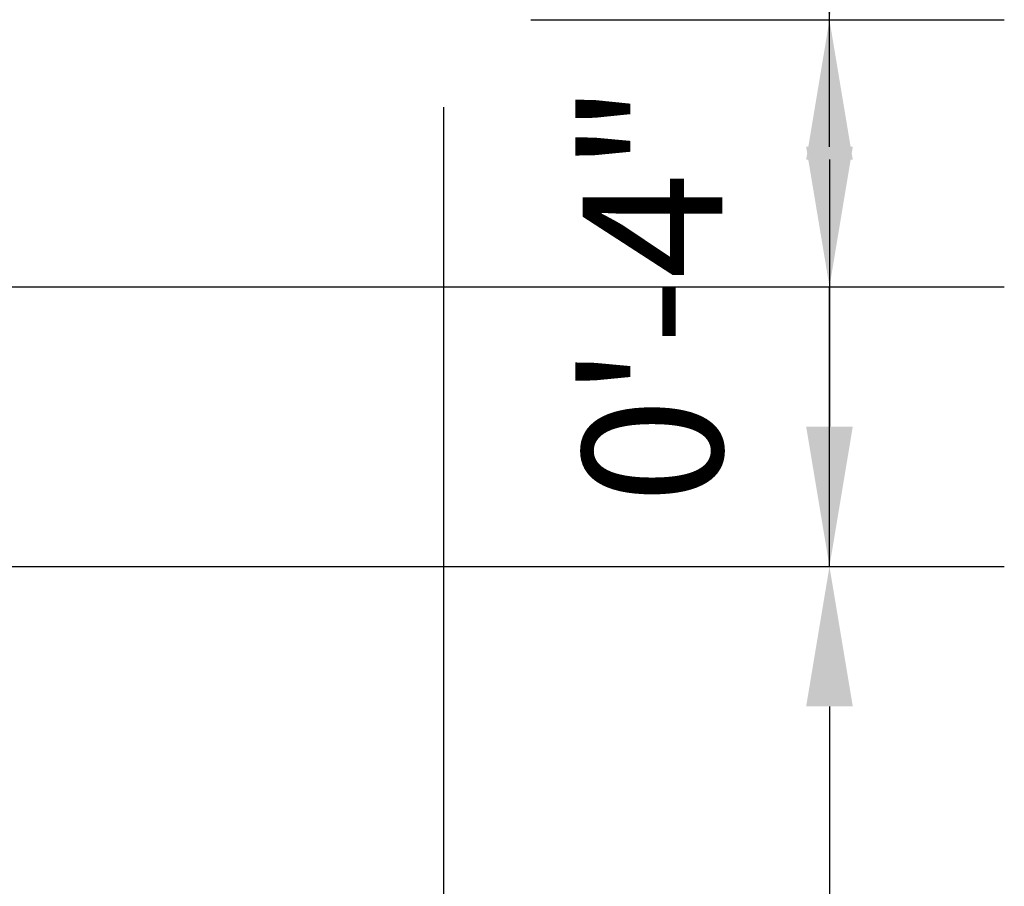
# Model space of a CAD drawing. Units: millimetres. Extents: x 7894 to 8038, y 6851 to 6951.
# Tile 36 of 49: x 7968.188 to 7975.227, y 6916.434 to 6922.628. Entities that reach past the tile are written whole.
import ezdxf

# ---------------------------------------------------------------- set-up
doc = ezdxf.new("R2010")
doc.units = ezdxf.units.MM
doc.layers.add('A-ANNO-DIMS', color=2, linetype='Continuous', lineweight=18)
doc.styles.get("Standard").update_dxf_attribs({"font": 'arial.ttf'})
doc.dimstyles.new('ISO-25', dxfattribs={"dimtxt": 1, "dimasz": 1, "dimexe": 1.25, "dimexo": 0.625, "dimtad": 1, "dimdec": 0, "dimlunit": 4, "dimtxsty": 'Standard', "dimcen": 2.5, "dimclrt": 1, "dimadec": 0, "dimazin": 0, "dimtfac": 1, "dimtdec": 0, "dimtmove": 0, "dimatfit": 3, "dimfxl": 1, "dimarcsym": 0})

# ---------------------------------------------------------------- blocks, each defined once
blk = doc.blocks.new('*D23')
at = {"layer": 'A-ANNO-DIMS', "color": 0, "lineweight": -2, "transparency": 16777216}
for p, q in [((7940.0888, 6907.098), (7940.0888, 6947.7928)), ((7971.9356, 6928.989), (7971.9356, 6947.7928)), ((7941.0888, 6946.5428), (7970.9356, 6946.5428))]:
    blk.add_line(p, q, dxfattribs=at)
at = {"layer": 'A-ANNO-DIMS', "color": 0, "transparency": 16777216}
for points in [[(7941.0888, 6946.7095), (7941.0888, 6946.3762), (7940.0888, 6946.5428)], [(7970.9356, 6946.7095), (7970.9356, 6946.3762), (7971.9356, 6946.5428)]]:
    blk.add_solid(points, dxfattribs=at)
at = {"layer": 'Defpoints', "color": 0, "transparency": 16777216}
for p in [(7971.9356, 6946.5428), (7971.9356, 6928.364), (7940.0888, 6906.473)]:
    blk.add_point(p, dxfattribs=at)
at = {"layer": 'A-ANNO-DIMS', "color": 1, "transparency": 16777216, "insert": (7956.0122, 6947.6784), "char_height": 1, "attachment_point": 5}
blk.add_mtext('2\'-8"', dxfattribs=at)
blk = doc.blocks.new('*D26')
at = {"layer": 'A-ANNO-DIMS', "color": 0, "lineweight": -2, "transparency": 16777216}
for p, q in [((7950.9654, 6918.7198), (7975.2272, 6918.7198)), ((7973.9772, 6917.7198), (7973.9772, 6907.4734)), ((7964.9658, 6906.4734), (7975.2272, 6906.4734))]:
    blk.add_line(p, q, dxfattribs=at)
at = {"layer": 'A-ANNO-DIMS', "color": 0, "transparency": 16777216}
for points in [[(7973.8105, 6917.7198), (7974.1439, 6917.7198), (7973.9772, 6918.7198)], [(7973.8105, 6907.4734), (7974.1439, 6907.4734), (7973.9772, 6906.4734)]]:
    blk.add_solid(points, dxfattribs=at)
at = {"layer": 'Defpoints', "color": 0, "transparency": 16777216}
for p in [(7950.3404, 6918.7198), (7964.3408, 6906.4734), (7973.9772, 6906.4734)]:
    blk.add_point(p, dxfattribs=at)
at = {"layer": 'A-ANNO-DIMS', "color": 1, "transparency": 16777216, "insert": (7972.8416, 6912.5966), "char_height": 1, "attachment_point": 5, "rotation": 90}
blk.add_mtext('1\'-0"', dxfattribs=at)
blk = doc.blocks.new('*D27')
at = {"layer": 'A-ANNO-DIMS', "color": 0, "lineweight": -2, "transparency": 16777216}
for p, q in [((7971.8421, 6922.6283), (7975.2272, 6922.6283)), ((7973.9772, 6921.6283), (7973.9772, 6919.7198)), ((7950.9654, 6918.7198), (7975.2272, 6918.7198))]:
    blk.add_line(p, q, dxfattribs=at)
at = {"layer": 'A-ANNO-DIMS', "color": 0, "transparency": 16777216}
for points in [[(7973.8105, 6921.6283), (7974.1439, 6921.6283), (7973.9772, 6922.6283)], [(7973.8105, 6919.7198), (7974.1439, 6919.7198), (7973.9772, 6918.7198)]]:
    blk.add_solid(points, dxfattribs=at)
at = {"layer": 'Defpoints', "color": 0, "transparency": 16777216}
for p in [(7971.2171, 6922.6283), (7950.3404, 6918.7198), (7973.9772, 6918.7198)]:
    blk.add_point(p, dxfattribs=at)
at = {"layer": 'A-ANNO-DIMS', "color": 1, "transparency": 16777216, "insert": (7972.8416, 6920.6741), "char_height": 1, "attachment_point": 5, "rotation": 90}
blk.add_mtext('0\'-4"', dxfattribs=at)
blk = doc.blocks.new('*D28')
at = {"layer": 'A-ANNO-DIMS', "color": 0, "lineweight": -2, "transparency": 16777216}
for p, q in [((7960.8854, 6936.8804), (7975.2272, 6936.8804)), ((7973.9772, 6935.8804), (7973.9772, 6923.6283)), ((7971.8421, 6922.6283), (7975.2272, 6922.6283))]:
    blk.add_line(p, q, dxfattribs=at)
at = {"layer": 'A-ANNO-DIMS', "color": 0, "transparency": 16777216}
for points in [[(7973.8105, 6935.8804), (7974.1439, 6935.8804), (7973.9772, 6936.8804)], [(7973.8105, 6923.6283), (7974.1439, 6923.6283), (7973.9772, 6922.6283)]]:
    blk.add_solid(points, dxfattribs=at)
at = {"layer": 'Defpoints', "color": 0, "transparency": 16777216}
for p in [(7960.2604, 6936.8804), (7971.2171, 6922.6283), (7973.9772, 6922.6283)]:
    blk.add_point(p, dxfattribs=at)
at = {"layer": 'A-ANNO-DIMS', "color": 1, "transparency": 16777216, "insert": (7972.8351, 6929.7543), "char_height": 1, "attachment_point": 5, "rotation": 90}
blk.add_mtext('1\'-2 1/2"', dxfattribs=at)
blk = doc.blocks.new('*D31')
at = {"layer": 'A-ANNO-DIMS', "color": 0, "lineweight": -2, "transparency": 16777216}
for p, q in [((7973.9772, 6921.7198), (7973.9772, 6926.628)), ((7949.8107, 6920.7198), (7975.2272, 6920.7198)), ((7973.9772, 6918.7198), (7973.9772, 6920.7198)), ((7950.9654, 6918.7198), (7975.2272, 6918.7198)), ((7973.9772, 6917.7198), (7973.9772, 6916.7198))]:
    blk.add_line(p, q, dxfattribs=at)
at = {"layer": 'A-ANNO-DIMS', "color": 0, "transparency": 16777216}
for points in [[(7973.8105, 6921.7198), (7974.1439, 6921.7198), (7973.9772, 6920.7198)], [(7973.8105, 6917.7198), (7974.1439, 6917.7198), (7973.9772, 6918.7198)]]:
    blk.add_solid(points, dxfattribs=at)
at = {"layer": 'Defpoints', "color": 0, "transparency": 16777216}
for p in [(7949.1857, 6920.7198), (7973.9772, 6920.7198), (7950.3404, 6918.7198)]:
    blk.add_point(p, dxfattribs=at)
at = {"layer": 'A-ANNO-DIMS', "color": 1, "transparency": 16777216, "insert": (7972.8416, 6924.6739), "char_height": 1, "attachment_point": 5, "rotation": 90}
blk.add_mtext('0\'-2"', dxfattribs=at)
blk = doc.blocks.new('*D34')
at = {"layer": 'A-ANNO-DIMS', "color": 0, "lineweight": -2, "transparency": 16777216}
for p, q in [((7971.2171, 6922.0033), (7971.2171, 6903.2865)), ((7964.3408, 6905.8484), (7964.3408, 6903.2865)), ((7965.3408, 6904.5365), (7970.2171, 6904.5365))]:
    blk.add_line(p, q, dxfattribs=at)
at = {"layer": 'A-ANNO-DIMS', "color": 0, "transparency": 16777216}
for points in [[(7965.3408, 6904.7032), (7965.3408, 6904.3699), (7964.3408, 6904.5365)], [(7970.2171, 6904.7032), (7970.2171, 6904.3699), (7971.2171, 6904.5365)]]:
    blk.add_solid(points, dxfattribs=at)
at = {"layer": 'Defpoints', "color": 0, "transparency": 16777216}
for p in [(7971.2171, 6922.6283), (7964.3408, 6906.4734), (7971.2171, 6904.5365)]:
    blk.add_point(p, dxfattribs=at)
at = {"layer": 'A-ANNO-DIMS', "color": 1, "transparency": 16777216, "insert": (7967.779, 6905.6721), "char_height": 1, "attachment_point": 5}
blk.add_mtext('0\'-7"', dxfattribs=at)

msp = doc.modelspace()

# ---------------------------------------------------------------- dimensions: what is measured, and where the dimension line sits
at = {"layer": 'A-ANNO-DIMS'}
for base, p1, p2, picture, middle in [((7971.9356, 6946.5428), (7940.0888, 6906.473), (7971.9356, 6928.364), '*D23', (7956.0122, 6947.6784)), ((7971.2171, 6904.5365), (7964.3408, 6906.4734), (7971.2171, 6922.6283), '*D34', (7967.779, 6905.6721))]:
    dim = msp.add_linear_dim(base=base, p1=p1, p2=p2, dimstyle='ISO-25', override={"dimdec": 1, "dimlfac": 1, "dimrnd": 0, "dimzin": 1, "dimdsep": 46, "dimlunit": 4, "dimfrac": 2}, dxfattribs=at)
    dim.commit()
    dim.dimension.update_dxf_attribs({"geometry": picture, "text_midpoint": middle})
for base, p1, p2, picture, middle in [((7973.9772, 6922.6283), (7960.2604, 6936.8804), (7971.2171, 6922.6283), '*D28', (7972.8351, 6929.7543)), ((7973.9772, 6920.7198), (7950.3404, 6918.7198), (7949.1857, 6920.7198), '*D31', (7972.8416, 6924.6739)), ((7973.9772, 6918.7198), (7971.2171, 6922.6283), (7950.3404, 6918.7198), '*D27', (7972.8416, 6920.6741)), ((7973.9772, 6906.4734), (7950.3404, 6918.7198), (7964.3408, 6906.4734), '*D26', (7972.8416, 6912.5966))]:
    dim = msp.add_linear_dim(base=base, p1=p1, p2=p2, angle=90, dimstyle='ISO-25', override={"dimdec": 1, "dimlfac": 1, "dimrnd": 0, "dimzin": 1, "dimdsep": 46, "dimlunit": 4, "dimfrac": 2}, dxfattribs=at)
    dim.commit()
    dim.dimension.update_dxf_attribs({"geometry": picture, "text_midpoint": middle})

doc.saveas('drawing.dxf')
